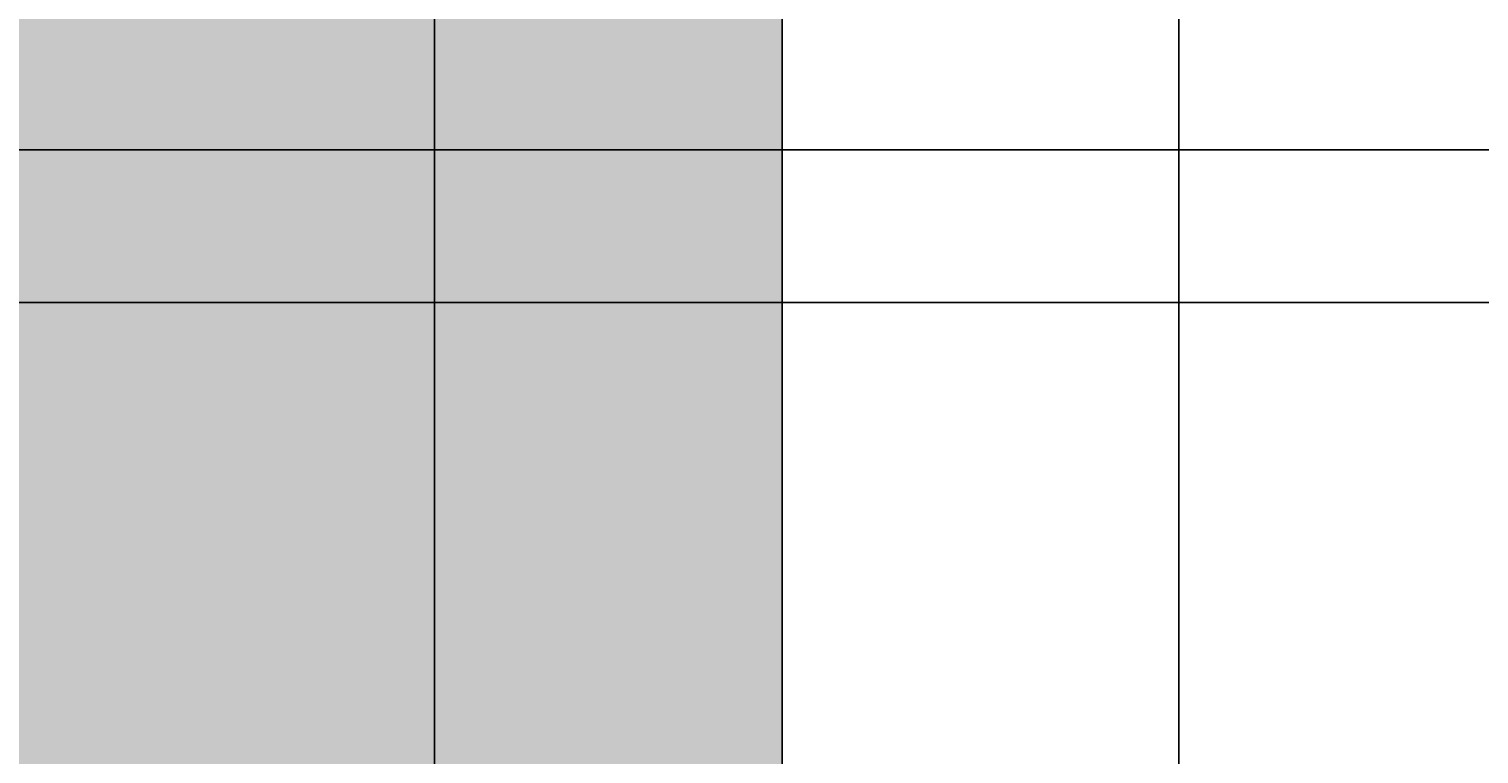
# Model space of a CAD drawing. Units: inches. Extents: x 35362 to 73946, y 43607 to 67532.
# Tile 61 of 134: x 47763 to 48533, y 47304 to 47689. Entities that reach past the tile are written whole.
import ezdxf

# ---------------------------------------------------------------- set-up
doc = ezdxf.new("R2010")
doc.units = ezdxf.units.IN
doc.header["$MEASUREMENT"] = 0
for name, color, linetype, lineweight in [('A-ANNO-DIMS', 2, 'Continuous', 18), ('E-SYMB', 1, 'Continuous', 25), ('E-SYMB-PATT', 1, 'Continuous', 13)]:
    doc.layers.add(name, color=color, linetype=linetype, lineweight=lineweight)
doc.styles.get("Standard").update_dxf_attribs({"font": 'arial.ttf'})
doc.dimstyles.get("Standard").update_dxf_attribs({"dimtxt": 0.18, "dimasz": 0.18, "dimexe": 0.18, "dimexo": 0.0625, "dimgap": 0.09, "dimtad": 0, "dimtih": 1, "dimtoh": 1, "dimdec": 4, "dimzin": 0, "dimdsep": 46, "dimtxsty": 'Standard', "dimcen": 0.09, "dimadec": 0, "dimazin": 0, "dimtfac": 1, "dimtdec": 4, "dimtofl": 0, "dimtmove": 0, "dimatfit": 3, "dimfxl": 1, "dimtolj": 1, "dimtzin": 0, "dimarcsym": 0})

# ---------------------------------------------------------------- blocks, each defined once
blk = doc.blocks.new('*D11')
at = {"layer": 'A-ANNO-DIMS', "color": 0, "lineweight": -2, "transparency": 16777216}
for p, q in [((47978.66, 56028.77), (47978.66, 43606.68)), ((53109.76, 56028.77), (53109.76, 43606.68)), ((47978.84, 43606.86), (50543.87, 43606.86)), ((53109.58, 43606.86), (50544.55, 43606.86))]:
    blk.add_line(p, q, dxfattribs=at)
at = {"layer": 'A-ANNO-DIMS', "color": 0, "transparency": 16777216}
for points in [[(47978.84, 43606.89), (47978.84, 43606.83), (47978.66, 43606.86)], [(53109.58, 43606.89), (53109.58, 43606.83), (53109.76, 43606.86)]]:
    blk.add_solid(points, dxfattribs=at)
at = {"layer": 'Defpoints', "color": 0, "transparency": 16777216}
for p in [(47978.66, 56028.84), (53109.76, 56028.84), (53109.76, 43606.86)]:
    blk.add_point(p, dxfattribs=at)
at = {"layer": 'A-ANNO-DIMS', "color": 0, "transparency": 16777216, "insert": (50544.21, 43606.86), "char_height": 0.18, "attachment_point": 5}
blk.add_mtext('\\A1;5131', dxfattribs=at)
blk = doc.blocks.new('*D13')
at = {"layer": 'A-ANNO-DIMS', "color": 0, "lineweight": -2, "transparency": 16777216}
for p, q in [((48373.49, 51694.02), (48373.49, 43606.68)), ((51029.04, 51694.02), (51029.04, 43606.68)), ((48373.67, 43606.86), (49700.8, 43606.86)), ((51028.86, 43606.86), (49701.73, 43606.86))]:
    blk.add_line(p, q, dxfattribs=at)
at = {"layer": 'A-ANNO-DIMS', "color": 0, "transparency": 16777216}
for points in [[(48373.67, 43606.89), (48373.67, 43606.83), (48373.49, 43606.86)], [(51028.86, 43606.89), (51028.86, 43606.83), (51029.04, 43606.86)]]:
    blk.add_solid(points, dxfattribs=at)
at = {"layer": 'Defpoints', "color": 0, "transparency": 16777216}
for p in [(48373.49, 51694.09), (51029.04, 51694.09), (51029.04, 43606.86)]:
    blk.add_point(p, dxfattribs=at)
at = {"layer": 'A-ANNO-DIMS', "color": 0, "transparency": 16777216, "insert": (49701.27, 43606.86), "char_height": 0.18, "attachment_point": 5}
blk.add_mtext('\\A1;2655.6', dxfattribs=at)
blk = doc.blocks.new('*D27')
at = {"layer": 'A-ANNO-DIMS', "color": 0, "lineweight": -2, "transparency": 16777216}
for p, q in [((47978.66, 56028.77), (47978.66, 43606.68)), ((48373.49, 53428.96), (48373.49, 43606.68)), ((47978.84, 43606.86), (48175.68, 43606.86)), ((48373.31, 43606.86), (48176.47, 43606.86))]:
    blk.add_line(p, q, dxfattribs=at)
at = {"layer": 'A-ANNO-DIMS', "color": 0, "transparency": 16777216}
for points in [[(47978.84, 43606.89), (47978.84, 43606.83), (47978.66, 43606.86)], [(48373.31, 43606.89), (48373.31, 43606.83), (48373.49, 43606.86)]]:
    blk.add_solid(points, dxfattribs=at)
at = {"layer": 'Defpoints', "color": 0, "transparency": 16777216}
for p in [(47978.66, 56028.84), (48373.49, 53429.02), (48373.49, 43606.86)]:
    blk.add_point(p, dxfattribs=at)
at = {"layer": 'A-ANNO-DIMS', "color": 0, "transparency": 16777216, "insert": (48176.08, 43606.86), "char_height": 0.18, "attachment_point": 5}
blk.add_mtext('\\A1;394.8', dxfattribs=at)
blk = doc.blocks.new('*D43')
at = {"layer": 'A-ANNO-DIMS', "color": 0, "lineweight": -2, "transparency": 16777216}
for p, q in [((62004.67, 47625.18), (35361.77, 47625.18)), ((35361.95, 47625), (35361.95, 47416.9)), ((35361.95, 47208.43), (35361.95, 47416.53)), ((62004.67, 47208.25), (35361.77, 47208.25))]:
    blk.add_line(p, q, dxfattribs=at)
at = {"layer": 'A-ANNO-DIMS', "color": 0, "transparency": 16777216}
for points in [[(35361.92, 47625), (35361.98, 47625), (35361.95, 47625.18)], [(35361.92, 47208.43), (35361.98, 47208.43), (35361.95, 47208.25)]]:
    blk.add_solid(points, dxfattribs=at)
at = {"layer": 'Defpoints', "color": 0, "transparency": 16777216}
for p in [(62004.73, 47625.18), (35361.95, 47208.25), (62004.73, 47208.25)]:
    blk.add_point(p, dxfattribs=at)
at = {"layer": 'A-ANNO-DIMS', "color": 0, "transparency": 16777216, "insert": (35361.95, 47416.72), "char_height": 0.18, "attachment_point": 5}
blk.add_mtext('\\A1;416.9', dxfattribs=at)
blk = doc.blocks.new('*D67')
at = {"layer": 'A-ANNO-DIMS', "color": 0, "lineweight": -2, "transparency": 16777216}
for p, q in [((56873.54, 53351.53), (35361.77, 53351.53)), ((35361.95, 53351.35), (35361.95, 49400.89)), ((35361.95, 45450.07), (35361.95, 49400.53)), ((53793.58, 45449.89), (35361.77, 45449.89))]:
    blk.add_line(p, q, dxfattribs=at)
at = {"layer": 'A-ANNO-DIMS', "color": 0, "transparency": 16777216}
for points in [[(35361.92, 53351.35), (35361.98, 53351.35), (35361.95, 53351.53)], [(35361.92, 45450.07), (35361.98, 45450.07), (35361.95, 45449.89)]]:
    blk.add_solid(points, dxfattribs=at)
at = {"layer": 'Defpoints', "color": 0, "transparency": 16777216}
for p in [(35361.95, 53351.53), (56873.6, 53351.53), (53793.64, 45449.89)]:
    blk.add_point(p, dxfattribs=at)
at = {"layer": 'A-ANNO-DIMS', "color": 0, "transparency": 16777216, "insert": (35361.95, 49400.71), "char_height": 0.18, "attachment_point": 5}
blk.add_mtext('\\A1;7901.6', dxfattribs=at)
blk = doc.blocks.new('*D87')
at = {"layer": 'A-ANNO-DIMS', "color": 0, "lineweight": -2, "transparency": 16777216}
for p, q in [((52362.49, 48318.27), (35361.77, 48318.27)), ((35361.95, 48318.09), (35361.95, 47931.38)), ((35361.95, 47544.31), (35361.95, 47931.02)), ((52362.49, 47544.13), (35361.77, 47544.13))]:
    blk.add_line(p, q, dxfattribs=at)
at = {"layer": 'A-ANNO-DIMS', "color": 0, "transparency": 16777216}
for points in [[(35361.92, 48318.09), (35361.98, 48318.09), (35361.95, 48318.27)], [(35361.92, 47544.31), (35361.98, 47544.31), (35361.95, 47544.13)]]:
    blk.add_solid(points, dxfattribs=at)
at = {"layer": 'Defpoints', "color": 0, "transparency": 16777216}
for p in [(35361.95, 48318.27), (52362.56, 48318.27), (52362.56, 47544.13)]:
    blk.add_point(p, dxfattribs=at)
at = {"layer": 'A-ANNO-DIMS', "color": 0, "transparency": 16777216, "insert": (35361.95, 47931.2), "char_height": 0.18, "attachment_point": 5}
blk.add_mtext('\\A1;774.1', dxfattribs=at)

msp = doc.modelspace()

# ---------------------------------------------------------------- hatches: boundary and pattern name
at = {"layer": 'E-SYMB-PATT'}
h = msp.add_hatch(color=256, dxfattribs=at)
h.dxf.hatch_style = 1
h.paths.add_polyline_path([(48163.038, 49689.843), (45390.147, 49689.843), (45390.147, 46919.381), (48163.038, 46919.381)])

# ---------------------------------------------------------------- linework, layer by layer
at = {"layer": 'E-SYMB'}
msp.add_lwpolyline([(45390.147, 49689.843), (48163.038, 49689.843), (48163.038, 46919.381), (45390.147, 46919.381)], close=True, dxfattribs=at)

# ---------------------------------------------------------------- dimensions: what is measured, and where the dimension line sits
at = {"layer": 'A-ANNO-DIMS'}
for base, p1, p2, override, picture, middle in [((53109.76, 43606.859), (47978.665, 56028.836), (53109.76, 56028.836), {"dimdec": 0, "dimlfac": 1, "dimrnd": 0, "dimzin": 0, "dimdsep": 46, "dimlunit": 2}, '*D11', (50544.212, 43606.859)), ((48373.492, 43606.859), (47978.665, 56028.836), (48373.492, 53429.019), {"dimdec": 1, "dimlfac": 1, "dimrnd": 0, "dimzin": 0, "dimdsep": 46, "dimlunit": 2}, '*D27', (48176.078, 43606.859)), ((51029.043, 43606.859), (48373.492, 51694.087), (51029.043, 51694.087), {"dimdec": 1, "dimlfac": 1, "dimrnd": 0, "dimzin": 0, "dimdsep": 46, "dimlunit": 2}, '*D13', (49701.267, 43606.859))]:
    dim = msp.add_linear_dim(base=base, p1=p1, p2=p2, dimstyle='Standard', override=override, dxfattribs=at)
    dim.commit()
    dim.dimension.update_dxf_attribs({"geometry": picture, "text_midpoint": middle})
for base, p1, p2, picture, middle in [((35361.949, 53351.529), (53793.638, 45449.894), (56873.602, 53351.529), '*D67', (35361.949, 49400.712)), ((35361.949, 48318.269), (52362.557, 47544.134), (52362.557, 48318.269), '*D87', (35361.949, 47931.201)), ((35361.949, 47208.25), (62004.728, 47625.181), (62004.728, 47208.25), '*D43', (35361.949, 47416.715))]:
    dim = msp.add_linear_dim(base=base, p1=p1, p2=p2, angle=90, dimstyle='Standard', override={"dimdec": 1, "dimlfac": 1, "dimrnd": 0, "dimzin": 0, "dimdsep": 46, "dimlunit": 2}, dxfattribs=at)
    dim.commit()
    dim.dimension.update_dxf_attribs({"geometry": picture, "text_midpoint": middle})

doc.saveas('drawing.dxf')
